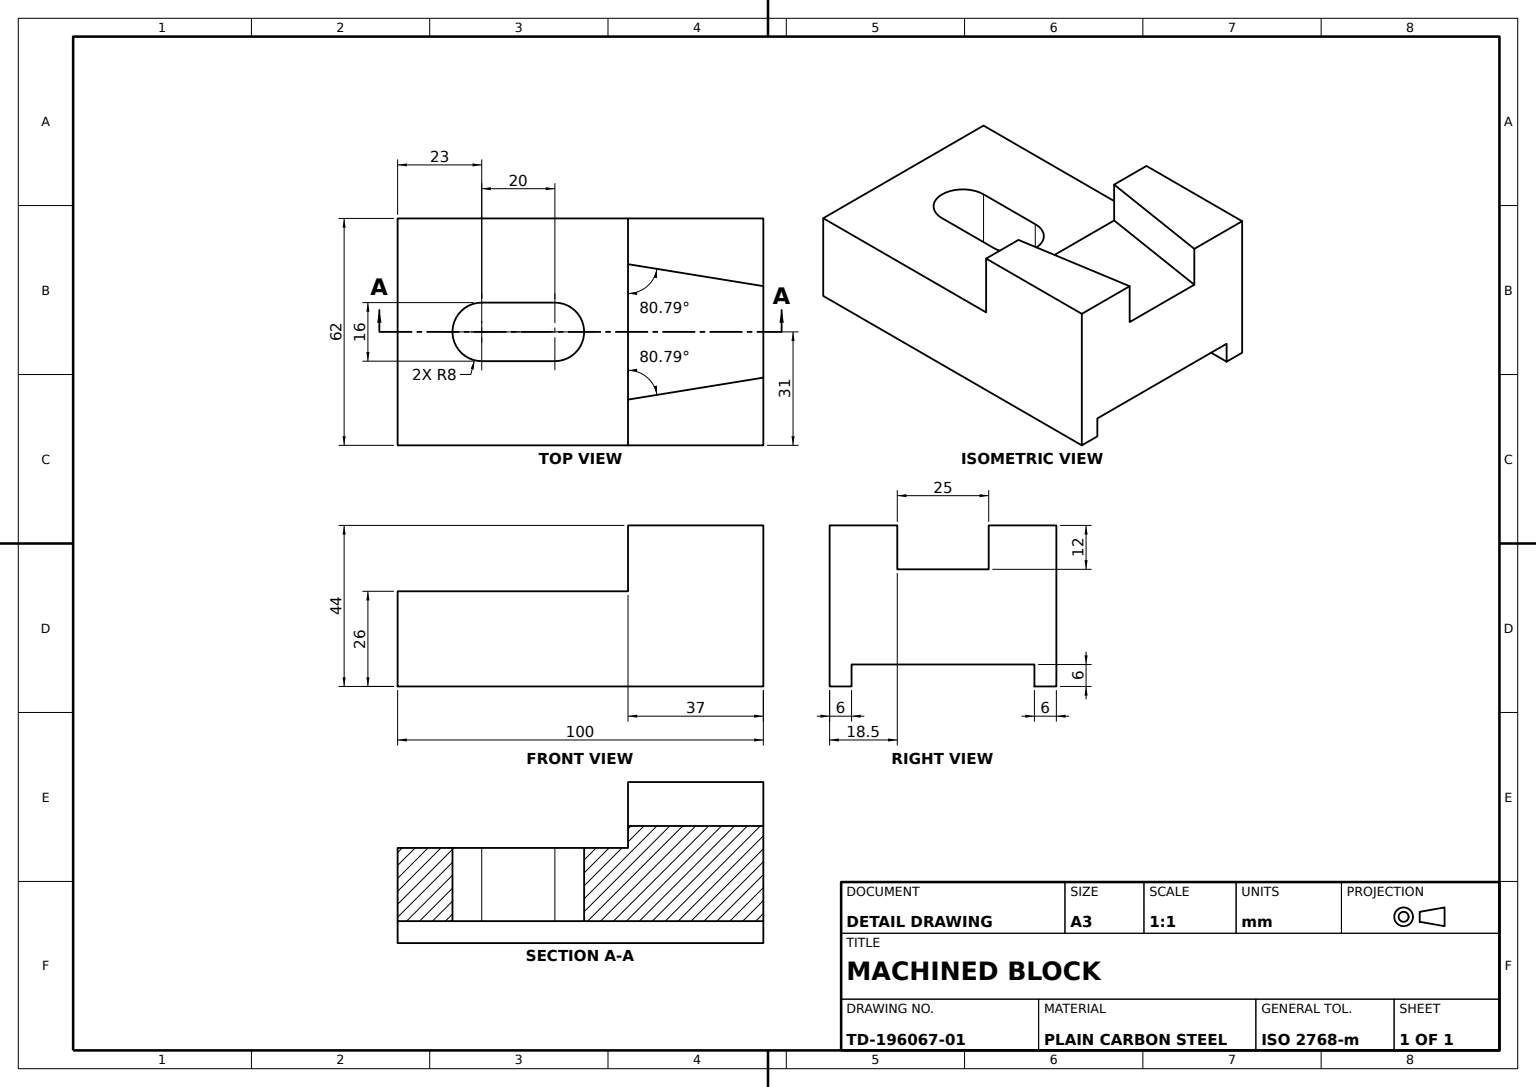
SolidWorks part; units mm, degrees
material "Plain Carbon Steel"
ref_plane "Front Plane" through (0, 0, 0) normal (0, 0, 1) x (1, 0, 0)
ref_plane "Top Plane" through (0, 0, 0) normal (0, 1, 0) x (1, 0, 0)
ref_plane "Right Plane" through (0, 0, 0) normal (1, 0, 0) x (0, 0, -1)
sketch "Base Profile Sketch" plane through (0, 0, 0) normal (0, 0, 1) x (1, 0, 0)
  line L0 (0, 99.2453) -> (0, -104.5283) construction
  line L1 (-172.956, 0) -> (196.6038, 0) construction
  line L2 (0, 0) -> (0, 26)
  line L3 (0, 26) -> (63, 26)
  line L4 (63, 26) -> (63, 44)
  line L5 (63, 44) -> (100, 44)
  line L6 (100, 44) -> (100, 0)
  line L7 (100, 0) -> (0, 0)
  dimension "D1" = 26
  dimension "D2" = 44
  dimension "D3" = 37
  dimension "D4" = 100
extrude "Base Block" add sketch "Base Profile Sketch" along normal mid plane 62
sketch "Stepped Channel Sketch" plane through (0, 26, 0) normal (0, 1, 0) x (1, 0, 0)
  line L0 (23, 0) -> (43, 0) construction
  line L1 (23, 8) -> (43, 8)
  line L2 (23, -8) -> (43, -8)
  line L3 (63, -31) -> (63, 31) construction
  arc A0 (23, 8) -> (23, -8) centre (23, 0) ccw
  arc A1 (43, -8) -> (43, 8) centre (43, 0) ccw
  point P3 (33, 0)
  dimension "D1" = 20
  dimension "D2" = 20
  dimension "D3" = 16
extrude "Stepped Channel Through" cut sketch "Stepped Channel Sketch" against normal blind 62
sketch "Top Slot Sketch" plane through (0, 44, 0) normal (0, 1, 0) x (1, 0, 0)
  line L0 (63, 18.5) -> (63, -18.5)
  line L1 (63, -31) -> (63, 31) construction
  line L2 (63, -31) -> (63, 31) construction
  line L3 (100, 12.5) -> (100, -12.5)
  line L4 (100, -31) -> (100, 31) construction
  line L5 (63, 18.5) -> (100, 12.5)
  line L6 (63, -18.5) -> (100, -12.5)
  line L7 (-19.9089, 0) -> (124.8546, 0) construction
  point P6 (63, 0)
  dimension "D1" = 18.5
  dimension "D2" = 25
extrude "Top Slot Pocket 12 Deep" cut sketch "Top Slot Sketch" against normal blind 12
sketch "Bottom Groove Sketch" plane through (0, 0, 0) normal (-1, 0, 0) x (0, 0, 1)
  line L1 (31, 0) -> (-31, 0) construction
  line L2 (-25, 0) -> (-25, 6)
  line L3 (-25, 6) -> (25, 6)
  line L4 (25, 6) -> (25, 0)
  line L5 (25, 0) -> (-25, 0)
  line L6 (-31, 26) -> (-31, 0) construction
  line L7 (31, 26) -> (31, 0) construction
  dimension "D1" = 6
  dimension "D2" = 6
  dimension "D3" = 6
extrude "Bottom Groove 6x6" cut sketch "Bottom Groove Sketch" against normal through all contours L3 L4 L5 L2
